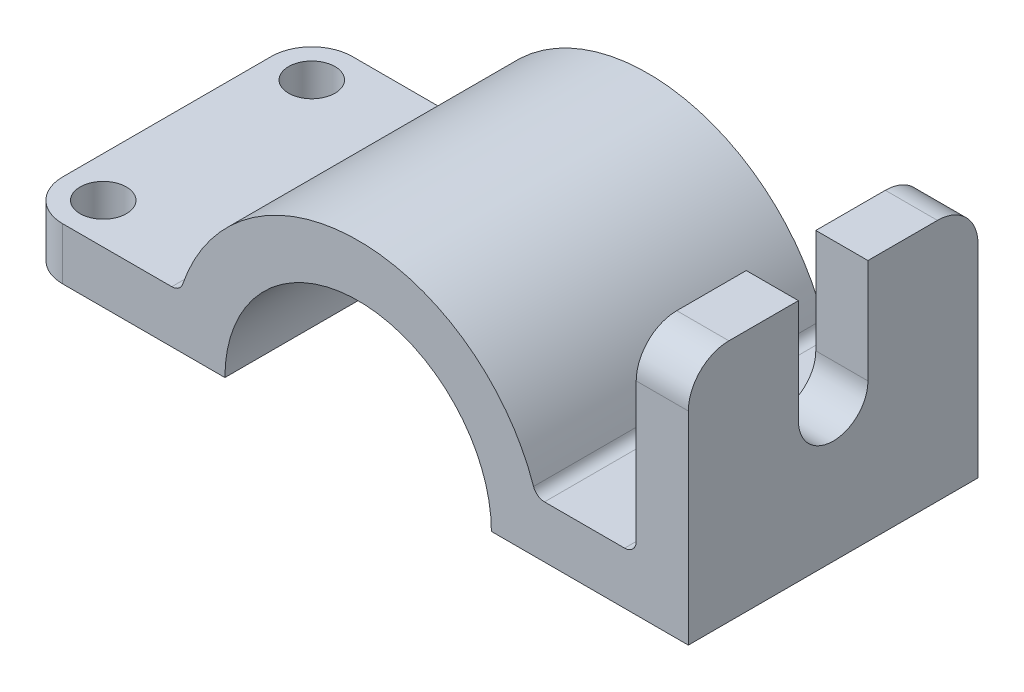
ISO-10303-21;
HEADER;
FILE_DESCRIPTION(('STEP AP214'),'2;1');
FILE_NAME('part.step','',(''),(''),'','','');
FILE_SCHEMA(('AUTOMOTIVE_DESIGN { 1 0 10303 214 1 1 1 1 }'));
ENDSEC;
DATA;
#1=APPLICATION_CONTEXT('core data for automotive mechanical design processes');
#2=APPLICATION_PROTOCOL_DEFINITION('international standard','automotive_design',2000,#1);
#3=PRODUCT_CONTEXT('',#1,'mechanical');
#4=PRODUCT('Part','Part','',(#3));
#5=PRODUCT_RELATED_PRODUCT_CATEGORY('part','',(#4));
#6=PRODUCT_DEFINITION_FORMATION('','',#4);
#7=PRODUCT_DEFINITION_CONTEXT('part definition',#1,'design');
#8=PRODUCT_DEFINITION('design','',#6,#7);
#9=PRODUCT_DEFINITION_SHAPE('','',#8);
#10=(LENGTH_UNIT() NAMED_UNIT(*) SI_UNIT(.MILLI.,.METRE.));
#11=(NAMED_UNIT(*) PLANE_ANGLE_UNIT() SI_UNIT($,.RADIAN.));
#12=(NAMED_UNIT(*) SI_UNIT($,.STERADIAN.) SOLID_ANGLE_UNIT());
#13=UNCERTAINTY_MEASURE_WITH_UNIT(LENGTH_MEASURE(1.E-05),#10,'distance_accuracy_value','');
#14=(GEOMETRIC_REPRESENTATION_CONTEXT(3) GLOBAL_UNCERTAINTY_ASSIGNED_CONTEXT((#13)) GLOBAL_UNIT_ASSIGNED_CONTEXT((#10,
#11,#12)) REPRESENTATION_CONTEXT('',''));
#15=CARTESIAN_POINT('',(0.,0.,0.));
#16=DIRECTION('',(0.,0.,1.));
#17=DIRECTION('',(1.,0.,0.));
#18=AXIS2_PLACEMENT_3D('',#15,#16,#17);
#19=CARTESIAN_POINT('',(57.,42.,25.));
#20=DIRECTION('',(0.,-1.,0.));
#21=DIRECTION('',(1.,0.,0.));
#22=AXIS2_PLACEMENT_3D('',#19,#20,#21);
#23=PLANE('',#22);
#24=DIRECTION('',(0.,0.,-1.));
#25=VECTOR('',#24,1.);
#26=CARTESIAN_POINT('',(57.,42.,25.));
#27=LINE('',#26,#25);
#28=CARTESIAN_POINT('',(57.,42.,18.));
#29=VERTEX_POINT('',#28);
#30=CARTESIAN_POINT('',(57.,42.,6.));
#31=VERTEX_POINT('',#30);
#32=EDGE_CURVE('E273',#29,#31,#27,.T.);
#33=ORIENTED_EDGE('',*,*,#32,.T.);
#34=DIRECTION('',(-1.,0.,0.));
#35=VECTOR('',#34,1.);
#36=CARTESIAN_POINT('',(57.,42.,6.));
#37=LINE('',#36,#35);
#38=CARTESIAN_POINT('',(48.,42.,6.));
#39=VERTEX_POINT('',#38);
#40=EDGE_CURVE('E209',#31,#39,#37,.T.);
#41=ORIENTED_EDGE('',*,*,#40,.T.);
#42=DIRECTION('',(0.,0.,-1.));
#43=VECTOR('',#42,1.);
#44=CARTESIAN_POINT('',(48.,42.,25.));
#45=LINE('',#44,#43);
#46=CARTESIAN_POINT('',(48.,42.,18.));
#47=VERTEX_POINT('',#46);
#48=EDGE_CURVE('E271',#47,#39,#45,.T.);
#49=ORIENTED_EDGE('',*,*,#48,.F.);
#50=DIRECTION('',(-1.,0.,0.));
#51=VECTOR('',#50,1.);
#52=CARTESIAN_POINT('',(57.,42.,18.));
#53=LINE('',#52,#51);
#54=EDGE_CURVE('E324',#47,#29,#53,.F.);
#55=ORIENTED_EDGE('',*,*,#54,.T.);
#56=EDGE_LOOP('',(#33,#41,#49,#55));
#57=FACE_BOUND('',#56,.T.);
#58=ADVANCED_FACE('F39',(#57),#23,.F.);
#59=CARTESIAN_POINT('',(0.,0.,25.));
#60=DIRECTION('',(0.,0.,-1.));
#61=DIRECTION('',(-1.,0.,0.));
#62=AXIS2_PLACEMENT_3D('',#59,#60,#61);
#63=CYLINDRICAL_SURFACE('',#62,23.);
#64=CARTESIAN_POINT('',(0.,0.,-25.));
#65=DIRECTION('',(0.,0.,-1.));
#66=DIRECTION('',(1.,0.,0.));
#67=AXIS2_PLACEMENT_3D('',#64,#65,#66);
#68=CIRCLE('',#67,23.);
#69=CARTESIAN_POINT('',(-23.,0.,-25.));
#70=VERTEX_POINT('',#69);
#71=CARTESIAN_POINT('',(23.,0.,-25.));
#72=VERTEX_POINT('',#71);
#73=EDGE_CURVE('E241',#70,#72,#68,.T.);
#74=ORIENTED_EDGE('',*,*,#73,.T.);
#75=DIRECTION('',(0.,0.,-1.));
#76=VECTOR('',#75,1.);
#77=CARTESIAN_POINT('',(23.,0.,25.));
#78=LINE('',#77,#76);
#79=CARTESIAN_POINT('',(23.,0.,25.));
#80=VERTEX_POINT('',#79);
#81=EDGE_CURVE('E278',#80,#72,#78,.T.);
#82=ORIENTED_EDGE('',*,*,#81,.F.);
#83=CARTESIAN_POINT('',(0.,0.,25.));
#84=DIRECTION('',(0.,0.,-1.));
#85=DIRECTION('',(1.,0.,0.));
#86=AXIS2_PLACEMENT_3D('',#83,#84,#85);
#87=CIRCLE('',#86,23.);
#88=CARTESIAN_POINT('',(-23.,0.,25.));
#89=VERTEX_POINT('',#88);
#90=EDGE_CURVE('E219',#89,#80,#87,.T.);
#91=ORIENTED_EDGE('',*,*,#90,.F.);
#92=DIRECTION('',(0.,0.,-1.));
#93=VECTOR('',#92,1.);
#94=CARTESIAN_POINT('',(-23.,0.,25.));
#95=LINE('',#94,#93);
#96=EDGE_CURVE('E245',#89,#70,#95,.T.);
#97=ORIENTED_EDGE('',*,*,#96,.T.);
#98=EDGE_LOOP('',(#74,#82,#91,#97));
#99=FACE_BOUND('',#98,.T.);
#100=ADVANCED_FACE('F421',(#99),#63,.F.);
#101=CARTESIAN_POINT('',(23.,0.,25.));
#102=DIRECTION('',(0.,1.,0.));
#103=DIRECTION('',(0.,0.,1.));
#104=AXIS2_PLACEMENT_3D('',#101,#102,#103);
#105=PLANE('',#104);
#106=DIRECTION('',(1.,0.,0.));
#107=VECTOR('',#106,1.);
#108=CARTESIAN_POINT('',(23.,0.,-25.));
#109=LINE('',#108,#107);
#110=CARTESIAN_POINT('',(57.,0.,-25.));
#111=VERTEX_POINT('',#110);
#112=EDGE_CURVE('E247',#72,#111,#109,.T.);
#113=ORIENTED_EDGE('',*,*,#112,.T.);
#114=DIRECTION('',(0.,0.,-1.));
#115=VECTOR('',#114,1.);
#116=CARTESIAN_POINT('',(57.,0.,25.));
#117=LINE('',#116,#115);
#118=CARTESIAN_POINT('',(57.,0.,25.));
#119=VERTEX_POINT('',#118);
#120=EDGE_CURVE('E280',#119,#111,#117,.T.);
#121=ORIENTED_EDGE('',*,*,#120,.F.);
#122=DIRECTION('',(1.,0.,0.));
#123=VECTOR('',#122,1.);
#124=CARTESIAN_POINT('',(23.,0.,25.));
#125=LINE('',#124,#123);
#126=EDGE_CURVE('E224',#80,#119,#125,.T.);
#127=ORIENTED_EDGE('',*,*,#126,.F.);
#128=ORIENTED_EDGE('',*,*,#81,.T.);
#129=EDGE_LOOP('',(#113,#121,#127,#128));
#130=FACE_BOUND('',#129,.T.);
#131=ADVANCED_FACE('F375',(#130),#105,.F.);
#132=CARTESIAN_POINT('',(57.,0.,25.));
#133=DIRECTION('',(-1.,0.,0.));
#134=DIRECTION('',(0.,0.,1.));
#135=AXIS2_PLACEMENT_3D('',#132,#133,#134);
#136=PLANE('',#135);
#137=CARTESIAN_POINT('',(57.,24.,0.));
#138=DIRECTION('',(1.,0.,0.));
#139=DIRECTION('',(0.,0.,-1.));
#140=AXIS2_PLACEMENT_3D('',#137,#138,#139);
#141=CIRCLE('',#140,6.);
#142=CARTESIAN_POINT('',(57.,24.,6.));
#143=VERTEX_POINT('',#142);
#144=CARTESIAN_POINT('',(57.,24.,-6.));
#145=VERTEX_POINT('',#144);
#146=EDGE_CURVE('E194',#143,#145,#141,.T.);
#147=ORIENTED_EDGE('',*,*,#146,.F.);
#148=DIRECTION('',(0.,-1.,0.));
#149=VECTOR('',#148,1.);
#150=CARTESIAN_POINT('',(57.,24.,6.));
#151=LINE('',#150,#149);
#152=EDGE_CURVE('E192',#31,#143,#151,.T.);
#153=ORIENTED_EDGE('',*,*,#152,.F.);
#154=ORIENTED_EDGE('',*,*,#32,.F.);
#155=CARTESIAN_POINT('',(57.,35.,18.));
#156=DIRECTION('',(-1.,0.,0.));
#157=DIRECTION('',(0.,0.,1.));
#158=AXIS2_PLACEMENT_3D('',#155,#156,#157);
#159=CIRCLE('',#158,7.);
#160=CARTESIAN_POINT('',(57.,35.,25.));
#161=VERTEX_POINT('',#160);
#162=EDGE_CURVE('E328',#29,#161,#159,.F.);
#163=ORIENTED_EDGE('',*,*,#162,.T.);
#164=DIRECTION('',(0.,1.,0.));
#165=VECTOR('',#164,1.);
#166=CARTESIAN_POINT('',(57.,0.,25.));
#167=LINE('',#166,#165);
#168=EDGE_CURVE('E228',#119,#161,#167,.T.);
#169=ORIENTED_EDGE('',*,*,#168,.F.);
#170=ORIENTED_EDGE('',*,*,#120,.T.);
#171=DIRECTION('',(0.,1.,0.));
#172=VECTOR('',#171,1.);
#173=CARTESIAN_POINT('',(57.,0.,-25.));
#174=LINE('',#173,#172);
#175=CARTESIAN_POINT('',(57.,35.,-25.));
#176=VERTEX_POINT('',#175);
#177=EDGE_CURVE('E249',#111,#176,#174,.T.);
#178=ORIENTED_EDGE('',*,*,#177,.T.);
#179=CARTESIAN_POINT('',(57.,35.,-18.));
#180=DIRECTION('',(-1.,0.,0.));
#181=DIRECTION('',(0.,0.,1.));
#182=AXIS2_PLACEMENT_3D('',#179,#180,#181);
#183=CIRCLE('',#182,7.);
#184=CARTESIAN_POINT('',(57.,42.,-18.));
#185=VERTEX_POINT('',#184);
#186=EDGE_CURVE('E330',#176,#185,#183,.F.);
#187=ORIENTED_EDGE('',*,*,#186,.T.);
#188=CARTESIAN_POINT('',(57.,42.,-6.));
#189=VERTEX_POINT('',#188);
#190=EDGE_CURVE('E204',#189,#185,#27,.T.);
#191=ORIENTED_EDGE('',*,*,#190,.F.);
#192=DIRECTION('',(0.,1.,0.));
#193=VECTOR('',#192,1.);
#194=CARTESIAN_POINT('',(57.,24.,-6.));
#195=LINE('',#194,#193);
#196=EDGE_CURVE('E188',#145,#189,#195,.T.);
#197=ORIENTED_EDGE('',*,*,#196,.F.);
#198=EDGE_LOOP('',(#147,#153,#154,#163,#169,#170,#178,#187,#191,#197));
#199=FACE_BOUND('',#198,.T.);
#200=ADVANCED_FACE('F205',(#199),#136,.F.);
#201=CARTESIAN_POINT('',(48.,42.,-6.));
#202=VERTEX_POINT('',#201);
#203=CARTESIAN_POINT('',(48.,42.,-18.));
#204=VERTEX_POINT('',#203);
#205=EDGE_CURVE('E269',#202,#204,#45,.T.);
#206=ORIENTED_EDGE('',*,*,#205,.F.);
#207=DIRECTION('',(1.,0.,0.));
#208=VECTOR('',#207,1.);
#209=CARTESIAN_POINT('',(57.,42.,-6.));
#210=LINE('',#209,#208);
#211=EDGE_CURVE('E53',#202,#189,#210,.T.);
#212=ORIENTED_EDGE('',*,*,#211,.T.);
#213=ORIENTED_EDGE('',*,*,#190,.T.);
#214=DIRECTION('',(-1.,0.,0.));
#215=VECTOR('',#214,1.);
#216=CARTESIAN_POINT('',(57.,42.,-18.));
#217=LINE('',#216,#215);
#218=EDGE_CURVE('E325',#185,#204,#217,.T.);
#219=ORIENTED_EDGE('',*,*,#218,.T.);
#220=EDGE_LOOP('',(#206,#212,#213,#219));
#221=FACE_BOUND('',#220,.T.);
#222=ADVANCED_FACE('F384',(#221),#23,.F.);
#223=CARTESIAN_POINT('',(48.,42.,25.));
#224=DIRECTION('',(1.,0.,0.));
#225=DIRECTION('',(0.,1.,0.));
#226=AXIS2_PLACEMENT_3D('',#223,#224,#225);
#227=PLANE('',#226);
#228=ORIENTED_EDGE('',*,*,#48,.T.);
#229=DIRECTION('',(0.,-1.,0.));
#230=VECTOR('',#229,1.);
#231=CARTESIAN_POINT('',(48.,42.,6.));
#232=LINE('',#231,#230);
#233=CARTESIAN_POINT('',(48.,24.,6.));
#234=VERTEX_POINT('',#233);
#235=EDGE_CURVE('E11',#39,#234,#232,.T.);
#236=ORIENTED_EDGE('',*,*,#235,.T.);
#237=CARTESIAN_POINT('',(48.,24.,0.));
#238=DIRECTION('',(1.,0.,0.));
#239=DIRECTION('',(0.,1.,0.));
#240=AXIS2_PLACEMENT_3D('',#237,#238,#239);
#241=CIRCLE('',#240,6.);
#242=CARTESIAN_POINT('',(48.,24.,-6.));
#243=VERTEX_POINT('',#242);
#244=EDGE_CURVE('E50',#234,#243,#241,.T.);
#245=ORIENTED_EDGE('',*,*,#244,.T.);
#246=DIRECTION('',(0.,1.,0.));
#247=VECTOR('',#246,1.);
#248=CARTESIAN_POINT('',(48.,42.,-6.));
#249=LINE('',#248,#247);
#250=EDGE_CURVE('E190',#243,#202,#249,.T.);
#251=ORIENTED_EDGE('',*,*,#250,.T.);
#252=ORIENTED_EDGE('',*,*,#205,.T.);
#253=CARTESIAN_POINT('',(48.,35.,-18.));
#254=DIRECTION('',(1.,0.,0.));
#255=DIRECTION('',(0.,1.,0.));
#256=AXIS2_PLACEMENT_3D('',#253,#254,#255);
#257=CIRCLE('',#256,7.);
#258=CARTESIAN_POINT('',(48.,35.,-25.));
#259=VERTEX_POINT('',#258);
#260=EDGE_CURVE('E318',#204,#259,#257,.F.);
#261=ORIENTED_EDGE('',*,*,#260,.T.);
#262=DIRECTION('',(0.,-1.,0.));
#263=VECTOR('',#262,1.);
#264=CARTESIAN_POINT('',(48.,42.,-25.));
#265=LINE('',#264,#263);
#266=CARTESIAN_POINT('',(48.,11.,-25.));
#267=VERTEX_POINT('',#266);
#268=EDGE_CURVE('E252',#259,#267,#265,.T.);
#269=ORIENTED_EDGE('',*,*,#268,.T.);
#270=DIRECTION('',(0.,0.,-1.));
#271=VECTOR('',#270,1.);
#272=CARTESIAN_POINT('',(48.,11.,25.));
#273=LINE('',#272,#271);
#274=CARTESIAN_POINT('',(48.,11.,25.));
#275=VERTEX_POINT('',#274);
#276=EDGE_CURVE('E288',#267,#275,#273,.F.);
#277=ORIENTED_EDGE('',*,*,#276,.T.);
#278=DIRECTION('',(0.,-1.,0.));
#279=VECTOR('',#278,1.);
#280=CARTESIAN_POINT('',(48.,42.,25.));
#281=LINE('',#280,#279);
#282=CARTESIAN_POINT('',(48.,35.,25.));
#283=VERTEX_POINT('',#282);
#284=EDGE_CURVE('E227',#283,#275,#281,.T.);
#285=ORIENTED_EDGE('',*,*,#284,.F.);
#286=CARTESIAN_POINT('',(48.,35.,18.));
#287=DIRECTION('',(1.,0.,0.));
#288=DIRECTION('',(0.,1.,0.));
#289=AXIS2_PLACEMENT_3D('',#286,#287,#288);
#290=CIRCLE('',#289,7.);
#291=EDGE_CURVE('E319',#283,#47,#290,.F.);
#292=ORIENTED_EDGE('',*,*,#291,.T.);
#293=EDGE_LOOP('',(#228,#236,#245,#251,#252,#261,#269,#277,#285,#292));
#294=FACE_BOUND('',#293,.T.);
#295=ADVANCED_FACE('F355',(#294),#227,.F.);
#296=CARTESIAN_POINT('',(48.,9.00000000000003,25.));
#297=DIRECTION('',(0.,-1.,0.));
#298=DIRECTION('',(1.,0.,0.));
#299=AXIS2_PLACEMENT_3D('',#296,#297,#298);
#300=PLANE('',#299);
#301=DIRECTION('',(-1.,0.,0.));
#302=VECTOR('',#301,1.);
#303=CARTESIAN_POINT('',(48.,9.00000000000003,25.));
#304=LINE('',#303,#302);
#305=CARTESIAN_POINT('',(46.,9.00000000000002,25.));
#306=VERTEX_POINT('',#305);
#307=CARTESIAN_POINT('',(32.1714158842908,9.,25.));
#308=VERTEX_POINT('',#307);
#309=EDGE_CURVE('E232',#306,#308,#304,.T.);
#310=ORIENTED_EDGE('',*,*,#309,.F.);
#311=DIRECTION('',(0.,0.,-1.));
#312=VECTOR('',#311,1.);
#313=CARTESIAN_POINT('',(46.,9.00000000000002,-25.));
#314=LINE('',#313,#312);
#315=CARTESIAN_POINT('',(46.,9.00000000000002,-25.));
#316=VERTEX_POINT('',#315);
#317=EDGE_CURVE('E284',#306,#316,#314,.T.);
#318=ORIENTED_EDGE('',*,*,#317,.T.);
#319=DIRECTION('',(-1.,0.,0.));
#320=VECTOR('',#319,1.);
#321=CARTESIAN_POINT('',(48.,9.00000000000003,-25.));
#322=LINE('',#321,#320);
#323=CARTESIAN_POINT('',(32.1714158842908,9.,-25.));
#324=VERTEX_POINT('',#323);
#325=EDGE_CURVE('E255',#316,#324,#322,.T.);
#326=ORIENTED_EDGE('',*,*,#325,.T.);
#327=DIRECTION('',(0.,0.,1.));
#328=VECTOR('',#327,1.);
#329=CARTESIAN_POINT('',(32.1714158842908,9.,25.));
#330=LINE('',#329,#328);
#331=EDGE_CURVE('E281',#324,#308,#330,.T.);
#332=ORIENTED_EDGE('',*,*,#331,.T.);
#333=EDGE_LOOP('',(#310,#318,#326,#332));
#334=FACE_BOUND('',#333,.T.);
#335=ADVANCED_FACE('F394',(#334),#300,.F.);
#336=CARTESIAN_POINT('',(0.,0.,25.));
#337=DIRECTION('',(0.,0.,-1.));
#338=DIRECTION('',(-1.,0.,0.));
#339=AXIS2_PLACEMENT_3D('',#336,#337,#338);
#340=CYLINDRICAL_SURFACE('',#339,32.);
#341=CARTESIAN_POINT('',(0.,0.,25.));
#342=DIRECTION('',(0.,0.,1.));
#343=DIRECTION('',(1.,0.,0.));
#344=AXIS2_PLACEMENT_3D('',#341,#342,#343);
#345=CIRCLE('',#344,32.);
#346=CARTESIAN_POINT('',(30.2789796558031,10.3529411764706,25.));
#347=VERTEX_POINT('',#346);
#348=CARTESIAN_POINT('',(-30.2789796558031,10.3529411764706,25.));
#349=VERTEX_POINT('',#348);
#350=EDGE_CURVE('E234',#347,#349,#345,.T.);
#351=ORIENTED_EDGE('',*,*,#350,.F.);
#352=DIRECTION('',(0.,0.,-1.));
#353=VECTOR('',#352,1.);
#354=CARTESIAN_POINT('',(30.2789796558031,10.3529411764706,25.));
#355=LINE('',#354,#353);
#356=CARTESIAN_POINT('',(30.2789796558031,10.3529411764706,-25.));
#357=VERTEX_POINT('',#356);
#358=EDGE_CURVE('E291',#347,#357,#355,.T.);
#359=ORIENTED_EDGE('',*,*,#358,.T.);
#360=CARTESIAN_POINT('',(0.,0.,-25.));
#361=DIRECTION('',(0.,0.,1.));
#362=DIRECTION('',(1.,0.,0.));
#363=AXIS2_PLACEMENT_3D('',#360,#361,#362);
#364=CIRCLE('',#363,32.);
#365=CARTESIAN_POINT('',(-30.2789796558031,10.3529411764706,-25.));
#366=VERTEX_POINT('',#365);
#367=EDGE_CURVE('E260',#357,#366,#364,.T.);
#368=ORIENTED_EDGE('',*,*,#367,.T.);
#369=DIRECTION('',(0.,0.,-1.));
#370=VECTOR('',#369,1.);
#371=CARTESIAN_POINT('',(-30.2789796558031,10.3529411764706,25.));
#372=LINE('',#371,#370);
#373=EDGE_CURVE('E292',#366,#349,#372,.F.);
#374=ORIENTED_EDGE('',*,*,#373,.T.);
#375=EDGE_LOOP('',(#351,#359,#368,#374));
#376=FACE_BOUND('',#375,.T.);
#377=ADVANCED_FACE('F401',(#376),#340,.T.);
#378=CARTESIAN_POINT('',(-30.7083050655682,8.99999999999999,25.));
#379=DIRECTION('',(0.,-1.,0.));
#380=DIRECTION('',(1.,0.,0.));
#381=AXIS2_PLACEMENT_3D('',#378,#379,#380);
#382=PLANE('',#381);
#383=CARTESIAN_POINT('',(-51.,8.99999999999999,-18.));
#384=DIRECTION('',(0.,1.,0.));
#385=DIRECTION('',(-1.,0.,0.));
#386=AXIS2_PLACEMENT_3D('',#383,#384,#385);
#387=CIRCLE('',#386,4.00000000000001);
#388=CARTESIAN_POINT('',(-55.,8.99999999999999,-18.));
#389=VERTEX_POINT('',#388);
#390=EDGE_CURVE('E212',#389,#389,#387,.T.);
#391=ORIENTED_EDGE('',*,*,#390,.F.);
#392=EDGE_LOOP('',(#391));
#393=FACE_BOUND('',#392,.T.);
#394=CARTESIAN_POINT('',(-51.,8.99999999999999,18.));
#395=DIRECTION('',(0.,1.,0.));
#396=DIRECTION('',(-1.,0.,0.));
#397=AXIS2_PLACEMENT_3D('',#394,#395,#396);
#398=CIRCLE('',#397,4.00000000000001);
#399=CARTESIAN_POINT('',(-55.,8.99999999999999,18.));
#400=VERTEX_POINT('',#399);
#401=EDGE_CURVE('E213',#400,#400,#398,.T.);
#402=ORIENTED_EDGE('',*,*,#401,.F.);
#403=EDGE_LOOP('',(#402));
#404=FACE_BOUND('',#403,.T.);
#405=DIRECTION('',(-1.,0.,0.));
#406=VECTOR('',#405,1.);
#407=CARTESIAN_POINT('',(-30.7083050655682,8.99999999999999,-25.));
#408=LINE('',#407,#406);
#409=CARTESIAN_POINT('',(-32.1714158842908,8.99999999999999,-25.));
#410=VERTEX_POINT('',#409);
#411=CARTESIAN_POINT('',(-51.,8.99999999999999,-25.));
#412=VERTEX_POINT('',#411);
#413=EDGE_CURVE('E257',#410,#412,#408,.T.);
#414=ORIENTED_EDGE('',*,*,#413,.T.);
#415=CARTESIAN_POINT('',(-51.,8.99999999999999,-18.));
#416=DIRECTION('',(0.,-1.,0.));
#417=DIRECTION('',(1.,0.,0.));
#418=AXIS2_PLACEMENT_3D('',#415,#416,#417);
#419=CIRCLE('',#418,7.);
#420=CARTESIAN_POINT('',(-58.,8.99999999999999,-18.));
#421=VERTEX_POINT('',#420);
#422=EDGE_CURVE('E65',#412,#421,#419,.F.);
#423=ORIENTED_EDGE('',*,*,#422,.T.);
#424=DIRECTION('',(0.,0.,-1.));
#425=VECTOR('',#424,1.);
#426=CARTESIAN_POINT('',(-58.,8.99999999999999,25.));
#427=LINE('',#426,#425);
#428=CARTESIAN_POINT('',(-58.,8.99999999999999,18.));
#429=VERTEX_POINT('',#428);
#430=EDGE_CURVE('E268',#429,#421,#427,.T.);
#431=ORIENTED_EDGE('',*,*,#430,.F.);
#432=CARTESIAN_POINT('',(-51.,8.99999999999999,18.));
#433=DIRECTION('',(0.,-1.,0.));
#434=DIRECTION('',(1.,0.,0.));
#435=AXIS2_PLACEMENT_3D('',#432,#433,#434);
#436=CIRCLE('',#435,7.);
#437=CARTESIAN_POINT('',(-51.,8.99999999999999,25.));
#438=VERTEX_POINT('',#437);
#439=EDGE_CURVE('E344',#429,#438,#436,.F.);
#440=ORIENTED_EDGE('',*,*,#439,.T.);
#441=DIRECTION('',(-1.,0.,0.));
#442=VECTOR('',#441,1.);
#443=CARTESIAN_POINT('',(-30.7083050655682,8.99999999999999,25.));
#444=LINE('',#443,#442);
#445=CARTESIAN_POINT('',(-32.1714158842908,8.99999999999999,25.));
#446=VERTEX_POINT('',#445);
#447=EDGE_CURVE('E240',#446,#438,#444,.T.);
#448=ORIENTED_EDGE('',*,*,#447,.F.);
#449=DIRECTION('',(0.,0.,1.));
#450=VECTOR('',#449,1.);
#451=CARTESIAN_POINT('',(-32.1714158842908,8.99999999999999,-25.));
#452=LINE('',#451,#450);
#453=EDGE_CURVE('E298',#446,#410,#452,.F.);
#454=ORIENTED_EDGE('',*,*,#453,.T.);
#455=EDGE_LOOP('',(#414,#423,#431,#440,#448,#454));
#456=FACE_BOUND('',#455,.T.);
#457=ADVANCED_FACE('F412',(#393,#404,#456),#382,.F.);
#458=CARTESIAN_POINT('',(-58.,8.99999999999999,25.));
#459=DIRECTION('',(1.,0.,0.));
#460=DIRECTION('',(0.,1.,0.));
#461=AXIS2_PLACEMENT_3D('',#458,#459,#460);
#462=PLANE('',#461);
#463=ORIENTED_EDGE('',*,*,#430,.T.);
#464=DIRECTION('',(0.,-1.,0.));
#465=VECTOR('',#464,1.);
#466=CARTESIAN_POINT('',(-58.,8.99999999999999,-18.));
#467=LINE('',#466,#465);
#468=CARTESIAN_POINT('',(-58.,0.,-18.));
#469=VERTEX_POINT('',#468);
#470=EDGE_CURVE('E340',#421,#469,#467,.T.);
#471=ORIENTED_EDGE('',*,*,#470,.T.);
#472=DIRECTION('',(0.,0.,-1.));
#473=VECTOR('',#472,1.);
#474=CARTESIAN_POINT('',(-58.,0.,25.));
#475=LINE('',#474,#473);
#476=CARTESIAN_POINT('',(-58.,0.,18.));
#477=VERTEX_POINT('',#476);
#478=EDGE_CURVE('E264',#477,#469,#475,.T.);
#479=ORIENTED_EDGE('',*,*,#478,.F.);
#480=DIRECTION('',(0.,-1.,0.));
#481=VECTOR('',#480,1.);
#482=CARTESIAN_POINT('',(-58.,8.99999999999999,18.));
#483=LINE('',#482,#481);
#484=EDGE_CURVE('E333',#477,#429,#483,.F.);
#485=ORIENTED_EDGE('',*,*,#484,.T.);
#486=EDGE_LOOP('',(#463,#471,#479,#485));
#487=FACE_BOUND('',#486,.T.);
#488=ADVANCED_FACE('F427',(#487),#462,.F.);
#489=CARTESIAN_POINT('',(-58.,0.,25.));
#490=DIRECTION('',(0.,1.,0.));
#491=DIRECTION('',(-1.,0.,0.));
#492=AXIS2_PLACEMENT_3D('',#489,#490,#491);
#493=PLANE('',#492);
#494=CARTESIAN_POINT('',(-51.,0.,-18.));
#495=DIRECTION('',(0.,1.,0.));
#496=DIRECTION('',(-1.,0.,0.));
#497=AXIS2_PLACEMENT_3D('',#494,#495,#496);
#498=CIRCLE('',#497,4.00000000000001);
#499=CARTESIAN_POINT('',(-55.,0.,-18.));
#500=VERTEX_POINT('',#499);
#501=EDGE_CURVE('E250',#500,#500,#498,.T.);
#502=ORIENTED_EDGE('',*,*,#501,.T.);
#503=EDGE_LOOP('',(#502));
#504=FACE_BOUND('',#503,.T.);
#505=CARTESIAN_POINT('',(-51.,0.,18.));
#506=DIRECTION('',(0.,1.,0.));
#507=DIRECTION('',(-1.,0.,0.));
#508=AXIS2_PLACEMENT_3D('',#505,#506,#507);
#509=CIRCLE('',#508,4.00000000000001);
#510=CARTESIAN_POINT('',(-55.,0.,18.));
#511=VERTEX_POINT('',#510);
#512=EDGE_CURVE('E220',#511,#511,#509,.T.);
#513=ORIENTED_EDGE('',*,*,#512,.T.);
#514=EDGE_LOOP('',(#513));
#515=FACE_BOUND('',#514,.T.);
#516=ORIENTED_EDGE('',*,*,#478,.T.);
#517=CARTESIAN_POINT('',(-51.,0.,-18.));
#518=DIRECTION('',(0.,1.,0.));
#519=DIRECTION('',(-1.,0.,0.));
#520=AXIS2_PLACEMENT_3D('',#517,#518,#519);
#521=CIRCLE('',#520,7.);
#522=CARTESIAN_POINT('',(-51.,0.,-25.));
#523=VERTEX_POINT('',#522);
#524=EDGE_CURVE('E345',#469,#523,#521,.F.);
#525=ORIENTED_EDGE('',*,*,#524,.T.);
#526=DIRECTION('',(1.,0.,0.));
#527=VECTOR('',#526,1.);
#528=CARTESIAN_POINT('',(-58.,0.,-25.));
#529=LINE('',#528,#527);
#530=EDGE_CURVE('E221',#523,#70,#529,.T.);
#531=ORIENTED_EDGE('',*,*,#530,.T.);
#532=ORIENTED_EDGE('',*,*,#96,.F.);
#533=DIRECTION('',(1.,0.,0.));
#534=VECTOR('',#533,1.);
#535=CARTESIAN_POINT('',(-58.,0.,25.));
#536=LINE('',#535,#534);
#537=CARTESIAN_POINT('',(-51.,0.,25.));
#538=VERTEX_POINT('',#537);
#539=EDGE_CURVE('E238',#538,#89,#536,.T.);
#540=ORIENTED_EDGE('',*,*,#539,.F.);
#541=CARTESIAN_POINT('',(-51.,0.,18.));
#542=DIRECTION('',(0.,1.,0.));
#543=DIRECTION('',(-1.,0.,0.));
#544=AXIS2_PLACEMENT_3D('',#541,#542,#543);
#545=CIRCLE('',#544,7.);
#546=EDGE_CURVE('E339',#538,#477,#545,.F.);
#547=ORIENTED_EDGE('',*,*,#546,.T.);
#548=EDGE_LOOP('',(#516,#525,#531,#532,#540,#547));
#549=FACE_BOUND('',#548,.T.);
#550=ADVANCED_FACE('F420',(#504,#515,#549),#493,.F.);
#551=CARTESIAN_POINT('',(0.,0.,25.));
#552=DIRECTION('',(0.,0.,1.));
#553=DIRECTION('',(1.,0.,0.));
#554=AXIS2_PLACEMENT_3D('',#551,#552,#553);
#555=PLANE('',#554);
#556=ORIENTED_EDGE('',*,*,#168,.T.);
#557=DIRECTION('',(-1.,0.,0.));
#558=VECTOR('',#557,1.);
#559=CARTESIAN_POINT('',(48.,35.,25.));
#560=LINE('',#559,#558);
#561=EDGE_CURVE('E312',#161,#283,#560,.T.);
#562=ORIENTED_EDGE('',*,*,#561,.T.);
#563=ORIENTED_EDGE('',*,*,#284,.T.);
#564=CARTESIAN_POINT('',(46.,11.,25.));
#565=DIRECTION('',(0.,0.,1.));
#566=DIRECTION('',(1.,0.,0.));
#567=AXIS2_PLACEMENT_3D('',#564,#565,#566);
#568=CIRCLE('',#567,2.);
#569=EDGE_CURVE('E305',#275,#306,#568,.F.);
#570=ORIENTED_EDGE('',*,*,#569,.T.);
#571=ORIENTED_EDGE('',*,*,#309,.T.);
#572=CARTESIAN_POINT('',(32.1714158842908,11.,25.));
#573=DIRECTION('',(0.,0.,1.));
#574=DIRECTION('',(1.,0.,0.));
#575=AXIS2_PLACEMENT_3D('',#572,#573,#574);
#576=CIRCLE('',#575,2.);
#577=EDGE_CURVE('E308',#308,#347,#576,.F.);
#578=ORIENTED_EDGE('',*,*,#577,.T.);
#579=ORIENTED_EDGE('',*,*,#350,.T.);
#580=CARTESIAN_POINT('',(-32.1714158842908,11.,25.));
#581=DIRECTION('',(0.,0.,1.));
#582=DIRECTION('',(1.,0.,0.));
#583=AXIS2_PLACEMENT_3D('',#580,#581,#582);
#584=CIRCLE('',#583,2.);
#585=EDGE_CURVE('E309',#349,#446,#584,.F.);
#586=ORIENTED_EDGE('',*,*,#585,.T.);
#587=ORIENTED_EDGE('',*,*,#447,.T.);
#588=DIRECTION('',(0.,-1.,0.));
#589=VECTOR('',#588,1.);
#590=CARTESIAN_POINT('',(-51.,0.,25.));
#591=LINE('',#590,#589);
#592=EDGE_CURVE('E315',#438,#538,#591,.T.);
#593=ORIENTED_EDGE('',*,*,#592,.T.);
#594=ORIENTED_EDGE('',*,*,#539,.T.);
#595=ORIENTED_EDGE('',*,*,#90,.T.);
#596=ORIENTED_EDGE('',*,*,#126,.T.);
#597=EDGE_LOOP('',(#556,#562,#563,#570,#571,#578,#579,#586,#587,#593,#594,#595,#596));
#598=FACE_BOUND('',#597,.T.);
#599=ADVANCED_FACE('F368',(#598),#555,.T.);
#600=CARTESIAN_POINT('',(0.,0.,-25.));
#601=DIRECTION('',(0.,0.,1.));
#602=DIRECTION('',(1.,0.,0.));
#603=AXIS2_PLACEMENT_3D('',#600,#601,#602);
#604=PLANE('',#603);
#605=ORIENTED_EDGE('',*,*,#268,.F.);
#606=DIRECTION('',(-1.,0.,0.));
#607=VECTOR('',#606,1.);
#608=CARTESIAN_POINT('',(0.,35.,-25.));
#609=LINE('',#608,#607);
#610=EDGE_CURVE('E334',#259,#176,#609,.F.);
#611=ORIENTED_EDGE('',*,*,#610,.T.);
#612=ORIENTED_EDGE('',*,*,#177,.F.);
#613=ORIENTED_EDGE('',*,*,#112,.F.);
#614=ORIENTED_EDGE('',*,*,#73,.F.);
#615=ORIENTED_EDGE('',*,*,#530,.F.);
#616=DIRECTION('',(0.,-1.,0.));
#617=VECTOR('',#616,1.);
#618=CARTESIAN_POINT('',(-51.,0.,-25.));
#619=LINE('',#618,#617);
#620=EDGE_CURVE('E332',#523,#412,#619,.F.);
#621=ORIENTED_EDGE('',*,*,#620,.T.);
#622=ORIENTED_EDGE('',*,*,#413,.F.);
#623=CARTESIAN_POINT('',(-32.1714158842908,11.,-25.));
#624=DIRECTION('',(0.,0.,1.));
#625=DIRECTION('',(1.,0.,0.));
#626=AXIS2_PLACEMENT_3D('',#623,#624,#625);
#627=CIRCLE('',#626,2.);
#628=EDGE_CURVE('E306',#410,#366,#627,.T.);
#629=ORIENTED_EDGE('',*,*,#628,.T.);
#630=ORIENTED_EDGE('',*,*,#367,.F.);
#631=CARTESIAN_POINT('',(32.1714158842908,11.,-25.));
#632=DIRECTION('',(0.,0.,1.));
#633=DIRECTION('',(1.,0.,0.));
#634=AXIS2_PLACEMENT_3D('',#631,#632,#633);
#635=CIRCLE('',#634,2.);
#636=EDGE_CURVE('E304',#357,#324,#635,.T.);
#637=ORIENTED_EDGE('',*,*,#636,.T.);
#638=ORIENTED_EDGE('',*,*,#325,.F.);
#639=CARTESIAN_POINT('',(46.,11.,-25.));
#640=DIRECTION('',(0.,0.,1.));
#641=DIRECTION('',(1.,0.,0.));
#642=AXIS2_PLACEMENT_3D('',#639,#640,#641);
#643=CIRCLE('',#642,2.);
#644=EDGE_CURVE('E297',#316,#267,#643,.T.);
#645=ORIENTED_EDGE('',*,*,#644,.T.);
#646=EDGE_LOOP('',(#605,#611,#612,#613,#614,#615,#621,#622,#629,#630,#637,#638,#645));
#647=FACE_BOUND('',#646,.T.);
#648=ADVANCED_FACE('F380',(#647),#604,.F.);
#649=CARTESIAN_POINT('',(46.,11.,25.));
#650=DIRECTION('',(0.,0.,1.));
#651=DIRECTION('',(1.,0.,0.));
#652=AXIS2_PLACEMENT_3D('',#649,#650,#651);
#653=CYLINDRICAL_SURFACE('',#652,2.);
#654=ORIENTED_EDGE('',*,*,#569,.F.);
#655=ORIENTED_EDGE('',*,*,#276,.F.);
#656=ORIENTED_EDGE('',*,*,#644,.F.);
#657=ORIENTED_EDGE('',*,*,#317,.F.);
#658=EDGE_LOOP('',(#654,#655,#656,#657));
#659=FACE_BOUND('',#658,.T.);
#660=ADVANCED_FACE('F393',(#659),#653,.F.);
#661=CARTESIAN_POINT('',(32.1714158842908,11.,25.));
#662=DIRECTION('',(0.,0.,-1.));
#663=DIRECTION('',(-1.,0.,0.));
#664=AXIS2_PLACEMENT_3D('',#661,#662,#663);
#665=CYLINDRICAL_SURFACE('',#664,2.);
#666=ORIENTED_EDGE('',*,*,#577,.F.);
#667=ORIENTED_EDGE('',*,*,#331,.F.);
#668=ORIENTED_EDGE('',*,*,#636,.F.);
#669=ORIENTED_EDGE('',*,*,#358,.F.);
#670=EDGE_LOOP('',(#666,#667,#668,#669));
#671=FACE_BOUND('',#670,.T.);
#672=ADVANCED_FACE('F398',(#671),#665,.F.);
#673=CARTESIAN_POINT('',(-32.1714158842908,11.,25.));
#674=DIRECTION('',(0.,0.,-1.));
#675=DIRECTION('',(-1.,0.,0.));
#676=AXIS2_PLACEMENT_3D('',#673,#674,#675);
#677=CYLINDRICAL_SURFACE('',#676,2.);
#678=ORIENTED_EDGE('',*,*,#585,.F.);
#679=ORIENTED_EDGE('',*,*,#373,.F.);
#680=ORIENTED_EDGE('',*,*,#628,.F.);
#681=ORIENTED_EDGE('',*,*,#453,.F.);
#682=EDGE_LOOP('',(#678,#679,#680,#681));
#683=FACE_BOUND('',#682,.T.);
#684=ADVANCED_FACE('F410',(#683),#677,.F.);
#685=CARTESIAN_POINT('',(0.,35.,18.));
#686=DIRECTION('',(1.,0.,0.));
#687=DIRECTION('',(0.,1.,0.));
#688=AXIS2_PLACEMENT_3D('',#685,#686,#687);
#689=CYLINDRICAL_SURFACE('',#688,7.);
#690=ORIENTED_EDGE('',*,*,#162,.F.);
#691=ORIENTED_EDGE('',*,*,#54,.F.);
#692=ORIENTED_EDGE('',*,*,#291,.F.);
#693=ORIENTED_EDGE('',*,*,#561,.F.);
#694=EDGE_LOOP('',(#690,#691,#692,#693));
#695=FACE_BOUND('',#694,.T.);
#696=ADVANCED_FACE('F362',(#695),#689,.T.);
#697=CARTESIAN_POINT('',(57.,35.,-18.));
#698=DIRECTION('',(-1.,0.,0.));
#699=DIRECTION('',(0.,-1.,0.));
#700=AXIS2_PLACEMENT_3D('',#697,#698,#699);
#701=CYLINDRICAL_SURFACE('',#700,7.);
#702=ORIENTED_EDGE('',*,*,#186,.F.);
#703=ORIENTED_EDGE('',*,*,#610,.F.);
#704=ORIENTED_EDGE('',*,*,#260,.F.);
#705=ORIENTED_EDGE('',*,*,#218,.F.);
#706=EDGE_LOOP('',(#702,#703,#704,#705));
#707=FACE_BOUND('',#706,.T.);
#708=ADVANCED_FACE('F385',(#707),#701,.T.);
#709=CARTESIAN_POINT('',(-51.,8.99999999999999,-18.));
#710=DIRECTION('',(0.,-1.,0.));
#711=DIRECTION('',(1.,0.,0.));
#712=AXIS2_PLACEMENT_3D('',#709,#710,#711);
#713=CYLINDRICAL_SURFACE('',#712,7.);
#714=ORIENTED_EDGE('',*,*,#422,.F.);
#715=ORIENTED_EDGE('',*,*,#620,.F.);
#716=ORIENTED_EDGE('',*,*,#524,.F.);
#717=ORIENTED_EDGE('',*,*,#470,.F.);
#718=EDGE_LOOP('',(#714,#715,#716,#717));
#719=FACE_BOUND('',#718,.T.);
#720=ADVANCED_FACE('F426',(#719),#713,.T.);
#721=CARTESIAN_POINT('',(-51.,0.,18.));
#722=DIRECTION('',(0.,1.,0.));
#723=DIRECTION('',(-1.,0.,0.));
#724=AXIS2_PLACEMENT_3D('',#721,#722,#723);
#725=CYLINDRICAL_SURFACE('',#724,7.);
#726=ORIENTED_EDGE('',*,*,#439,.F.);
#727=ORIENTED_EDGE('',*,*,#484,.F.);
#728=ORIENTED_EDGE('',*,*,#546,.F.);
#729=ORIENTED_EDGE('',*,*,#592,.F.);
#730=EDGE_LOOP('',(#726,#727,#728,#729));
#731=FACE_BOUND('',#730,.T.);
#732=ADVANCED_FACE('F41',(#731),#725,.T.);
#733=CARTESIAN_POINT('',(-51.,-41.,18.));
#734=DIRECTION('',(0.,1.,0.));
#735=DIRECTION('',(-1.,0.,0.));
#736=AXIS2_PLACEMENT_3D('',#733,#734,#735);
#737=CYLINDRICAL_SURFACE('',#736,4.00000000000001);
#738=ORIENTED_EDGE('',*,*,#401,.T.);
#739=EDGE_LOOP('',(#738));
#740=FACE_BOUND('',#739,.T.);
#741=ORIENTED_EDGE('',*,*,#512,.F.);
#742=EDGE_LOOP('',(#741));
#743=FACE_BOUND('',#742,.T.);
#744=ADVANCED_FACE('F471',(#740,#743),#737,.F.);
#745=CARTESIAN_POINT('',(-51.,-41.,-18.));
#746=DIRECTION('',(0.,1.,0.));
#747=DIRECTION('',(-1.,0.,0.));
#748=AXIS2_PLACEMENT_3D('',#745,#746,#747);
#749=CYLINDRICAL_SURFACE('',#748,4.00000000000001);
#750=ORIENTED_EDGE('',*,*,#390,.T.);
#751=EDGE_LOOP('',(#750));
#752=FACE_BOUND('',#751,.T.);
#753=ORIENTED_EDGE('',*,*,#501,.F.);
#754=EDGE_LOOP('',(#753));
#755=FACE_BOUND('',#754,.T.);
#756=ADVANCED_FACE('F480',(#752,#755),#749,.F.);
#757=CARTESIAN_POINT('',(37.,24.,0.));
#758=DIRECTION('',(1.,0.,0.));
#759=DIRECTION('',(0.,0.,-1.));
#760=AXIS2_PLACEMENT_3D('',#757,#758,#759);
#761=CYLINDRICAL_SURFACE('',#760,6.);
#762=DIRECTION('',(1.,0.,0.));
#763=VECTOR('',#762,1.);
#764=CARTESIAN_POINT('',(37.,24.,6.));
#765=LINE('',#764,#763);
#766=EDGE_CURVE('E189',#234,#143,#765,.T.);
#767=ORIENTED_EDGE('',*,*,#766,.T.);
#768=ORIENTED_EDGE('',*,*,#146,.T.);
#769=DIRECTION('',(1.,0.,0.));
#770=VECTOR('',#769,1.);
#771=CARTESIAN_POINT('',(37.,24.,-6.));
#772=LINE('',#771,#770);
#773=EDGE_CURVE('E185',#243,#145,#772,.T.);
#774=ORIENTED_EDGE('',*,*,#773,.F.);
#775=ORIENTED_EDGE('',*,*,#244,.F.);
#776=EDGE_LOOP('',(#767,#768,#774,#775));
#777=FACE_BOUND('',#776,.T.);
#778=ADVANCED_FACE('F191',(#777),#761,.F.);
#779=CARTESIAN_POINT('',(37.,24.,6.));
#780=DIRECTION('',(0.,0.,1.));
#781=DIRECTION('',(1.,0.,0.));
#782=AXIS2_PLACEMENT_3D('',#779,#780,#781);
#783=PLANE('',#782);
#784=ORIENTED_EDGE('',*,*,#152,.T.);
#785=ORIENTED_EDGE('',*,*,#766,.F.);
#786=ORIENTED_EDGE('',*,*,#235,.F.);
#787=ORIENTED_EDGE('',*,*,#40,.F.);
#788=EDGE_LOOP('',(#784,#785,#786,#787));
#789=FACE_BOUND('',#788,.T.);
#790=ADVANCED_FACE('F354',(#789),#783,.F.);
#791=CARTESIAN_POINT('',(37.,24.,-6.));
#792=DIRECTION('',(0.,0.,-1.));
#793=DIRECTION('',(-1.,0.,0.));
#794=AXIS2_PLACEMENT_3D('',#791,#792,#793);
#795=PLANE('',#794);
#796=ORIENTED_EDGE('',*,*,#250,.F.);
#797=ORIENTED_EDGE('',*,*,#773,.T.);
#798=ORIENTED_EDGE('',*,*,#196,.T.);
#799=ORIENTED_EDGE('',*,*,#211,.F.);
#800=EDGE_LOOP('',(#796,#797,#798,#799));
#801=FACE_BOUND('',#800,.T.);
#802=ADVANCED_FACE('F184',(#801),#795,.F.);
#803=CLOSED_SHELL('',(#58,#100,#131,#200,#222,#295,#335,#377,#457,#488,#550,#599,#648,#660,#672,
#684,#696,#708,#720,#732,#744,#756,#778,#790,#802));
#804=MANIFOLD_SOLID_BREP('B2',#803);
#805=ADVANCED_BREP_SHAPE_REPRESENTATION('',(#18,#804),#14);
#806=SHAPE_DEFINITION_REPRESENTATION(#9,#805);
ENDSEC;
END-ISO-10303-21;
